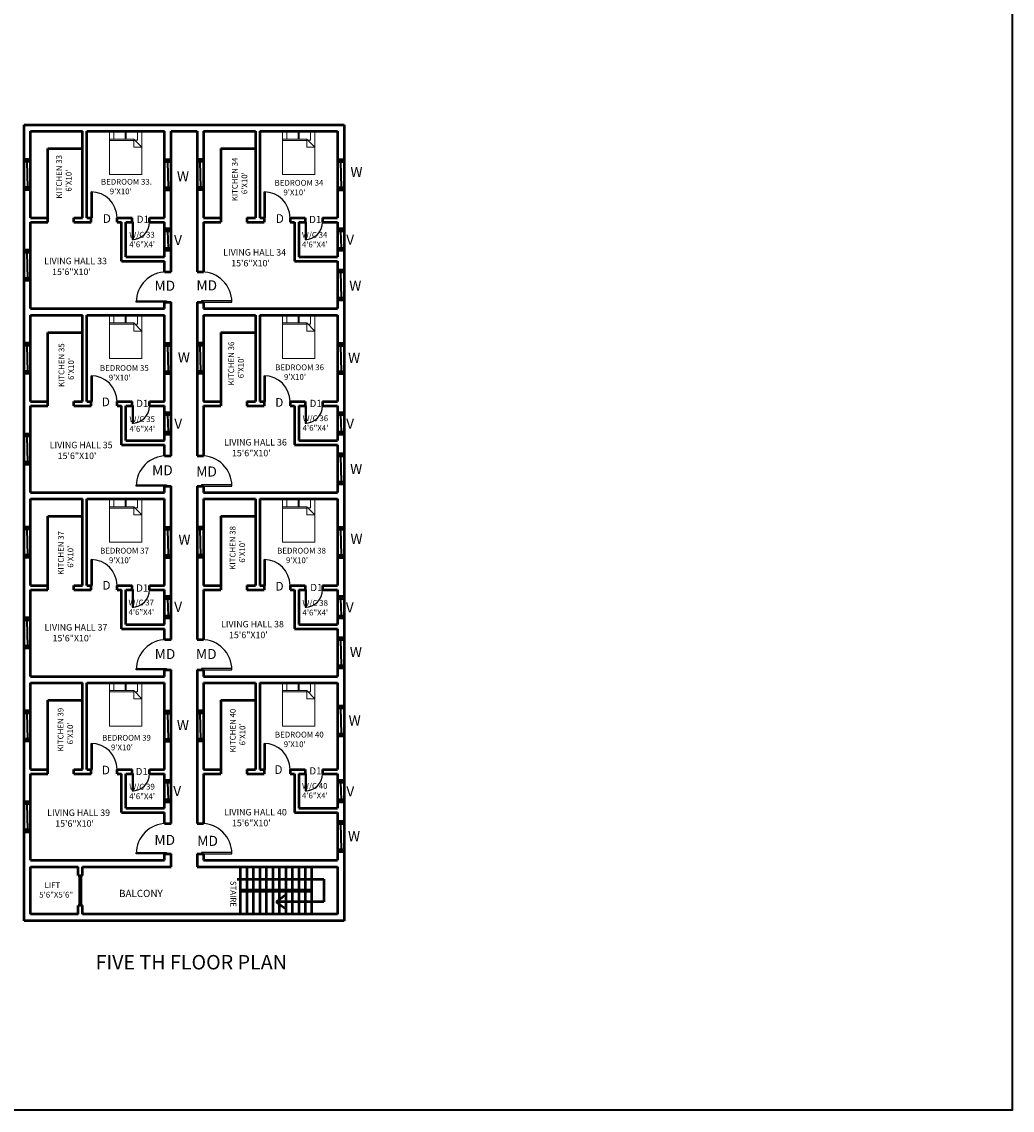
# Model space of a CAD drawing. Units: inches. Extents: x 9239 to 26065, y 6728 to 14611.
# Tile 9 of 12: x 24691 to 26065, y 11592 to 13102. Entities that reach past the tile are written whole.
import ezdxf

# ---------------------------------------------------------------- set-up
doc = ezdxf.new("R2010")
doc.units = ezdxf.units.IN
doc.header["$MEASUREMENT"] = 0
for name, color, linetype, lineweight in [('A-ANNO-TEXT', 7, 'Continuous', 18), ('A-ANNO-TTLB', 7, 'Continuous', 35), ('A-AREA-IDEN', 7, 'Continuous', 18), ('A-DOOR', 4, 'Continuous', 25), ('A-FURN', 8, 'Continuous', 18), ('A-GLAZ', 4, 'Continuous', 25), ('A-WALL', 7, 'Continuous', 50)]:
    doc.layers.add(name, color=color, linetype=linetype, lineweight=lineweight)
doc.styles.get("Standard").update_dxf_attribs({"font": 'arial.ttf'})

# ---------------------------------------------------------------- blocks, each defined once
blk = doc.blocks.new('*U10')
for p, q in [((0, 0), (0, -6)), ((36, 0), (36, -6))]:
    blk.add_line(p, q)
blk.add_lwpolyline([(0, 0), (0, 36), (1.75, 36), (1.75, 0)], close=True)
blk.add_arc((0, 0), 36, 0, 90)
blk = doc.blocks.new('*U34')
for p, q in [((0, 0), (0, 6)), ((24, 0), (24, 6))]:
    blk.add_line(p, q)
blk.add_lwpolyline([(0, 0), (0, -24), (1.75, -24), (1.75, 0)], close=True)
blk.add_arc((0, 0), 24, 270, 0)
blk = doc.blocks.new('*U33')
for p, q in [((-40, 0), (-40, 6)), ((0, 0), (0, 6))]:
    blk.add_line(p, q)
blk.add_lwpolyline([(0, 0), (0, -40), (-1.75, -40), (-1.75, 0)], close=True)
blk.add_arc((0, 0), 40, 180, 270)
blk = doc.blocks.new('*U35')
for p, q in [((0, 0), (0, -6)), ((-40, 0), (-40, -6))]:
    blk.add_line(p, q)
blk.add_lwpolyline([(0, 0), (0, 40), (-1.75, 40), (-1.75, 0)], close=True)
blk.add_arc((0, 0), 40, 90, 180)
blk = doc.blocks.new('Bed - Queen')
for p, q in [((0, -80.00003), (0, 0)), ((0, 0), (59.99999, 0)), ((59.99999, 0), (59.99999, -80.00003)), ((0, -14.4), (44.8, -14.4)), ((44.8, -16.8), (0, -16.8)), ((7.99999, -1.2), (28.79998, -1.2)), ((7.99999, -14.4), (7.99999, -1.2)), ((28.79998, -1.2), (28.79998, -14.4)), ((31.19999, -1.2), (51.99999, -1.2)), ((31.19999, -14.4), (31.19999, -1.2)), ((59.99999, -29.6), (44.8, -14.4)), ((44.8, -14.4), (44.8, -29.6)), ((51.99999, -16.4), (46.79936, -16.4)), ((51.99999, -1.2), (51.99999, -16.4)), ((44.8, -29.6), (59.99999, -29.6)), ((59.99999, -80.00003), (0, -80.00003))]:
    blk.add_line(p, q)
blk = doc.blocks.new('WIN-36')
for p, q in [((0, 1), (36, 1)), ((0, 0.5), (36, 0.5)), ((0, 0), (36, 0))]:
    blk.add_line(p, q)
blk = doc.blocks.new('WIN-24')
for p, q in [((0, 1), (24, 1)), ((0, 0.5), (24, 0.5)), ((0, 0), (24, 0))]:
    blk.add_line(p, q)

msp = doc.modelspace()

# ---------------------------------------------------------------- linework, layer by layer
at = {"layer": 'A-ANNO-TTLB'}
msp.add_lwpolyline([(23324.14, 14611.25), (26064.6, 14611.25), (26064.6, 11591.84), (23324.14, 11591.84)], close=True, dxfattribs=at)
at = {"layer": 'A-WALL'}
for p, q in [((24693.68, 12958.64), (25137.68, 12958.64)), ((24693.68, 11854.64), (24693.68, 12958.64)), ((25137.68, 12958.64), (25137.68, 11854.64)), ((24702.68, 12949.64), (24774.68, 12949.64)), ((24702.68, 12829.64), (24702.68, 12949.64)), ((24774.68, 12829.64), (24774.68, 12949.64)), ((24780.68, 12829.64), (24780.68, 12949.64)), ((24780.68, 12949.64), (24888.68, 12949.64)), ((24888.68, 12829.64), (24888.68, 12949.64)), ((24897.68, 12754.64), (24897.68, 12949.64)), ((24897.68, 12949.64), (24933.68, 12949.64)), ((24933.68, 12949.64), (24933.68, 12754.64)), ((24942.68, 12949.64), (24942.68, 12829.64)), ((24942.68, 12949.64), (25014.68, 12949.64)), ((25014.68, 12949.64), (25014.68, 12829.64)), ((25020.68, 12949.64), (25020.68, 12829.64)), ((25020.68, 12949.64), (25128.68, 12949.64)), ((25128.68, 12949.64), (25128.68, 12829.64)), ((24726.68, 12829.64), (24726.68, 12925.64)), ((24726.68, 12925.64), (24774.68, 12925.64)), ((24966.68, 12925.64), (24966.68, 12829.64)), ((24966.68, 12925.64), (25014.68, 12925.64)), ((24702.68, 12910.64), (24693.68, 12910.64)), ((24888.68, 12910.64), (24897.68, 12910.64)), ((24942.68, 12910.64), (24933.68, 12910.64)), ((25128.68, 12910.64), (25137.68, 12910.64)), ((24702.68, 12907.64), (24693.68, 12907.64)), ((24888.68, 12907.64), (24897.68, 12907.64)), ((24942.68, 12907.64), (24933.68, 12907.64)), ((25128.68, 12907.64), (25137.68, 12907.64)), ((24702.68, 12871.64), (24693.68, 12871.64)), ((24702.68, 12868.64), (24693.68, 12868.64)), ((24888.68, 12871.64), (24897.68, 12871.64)), ((24888.68, 12868.64), (24897.68, 12868.64)), ((24942.68, 12871.64), (24933.68, 12871.64)), ((24942.68, 12868.64), (24933.68, 12868.64)), ((25128.68, 12871.64), (25137.68, 12871.64)), ((25128.68, 12868.64), (25137.68, 12868.64)), ((24702.68, 12829.64), (24726.68, 12829.64)), ((24702.68, 12823.64), (24726.68, 12823.64)), ((24702.68, 12703.64), (24702.68, 12823.64)), ((24726.68, 12823.64), (24726.68, 12829.64)), ((24762.68, 12823.64), (24762.68, 12829.64)), ((24762.68, 12829.64), (24774.68, 12829.64)), ((24762.68, 12823.64), (24786.68, 12823.64)), ((24780.68, 12829.64), (24786.68, 12829.64)), ((24786.68, 12823.64), (24786.68, 12829.64)), ((24822.68, 12823.64), (24822.68, 12829.64)), ((24822.68, 12829.64), (24843.68, 12829.64)), ((24822.68, 12823.64), (24828.68, 12823.64)), ((24828.68, 12769.64), (24828.68, 12823.64)), ((24834.68, 12775.64), (24834.68, 12823.64)), ((24834.68, 12823.64), (24843.68, 12823.64)), ((24843.68, 12823.64), (24843.68, 12829.64)), ((24867.68, 12823.64), (24867.68, 12829.64)), ((24867.68, 12829.64), (24888.68, 12829.64)), ((24867.68, 12823.64), (24888.68, 12823.64)), ((24888.68, 12775.64), (24888.68, 12823.64)), ((24942.68, 12829.64), (24966.68, 12829.64)), ((24942.68, 12823.64), (24966.68, 12823.64)), ((24942.68, 12823.64), (24942.68, 12754.64)), ((24966.68, 12829.64), (24966.68, 12823.64)), ((25002.68, 12829.64), (25002.68, 12823.64)), ((25002.68, 12829.64), (25014.68, 12829.64)), ((25002.68, 12823.64), (25026.68, 12823.64)), ((25020.68, 12829.64), (25026.68, 12829.64)), ((25026.68, 12829.64), (25026.68, 12823.64)), ((25062.68, 12829.64), (25062.68, 12823.64)), ((25062.68, 12829.64), (25083.68, 12829.64)), ((25062.68, 12823.64), (25068.68, 12823.64)), ((25068.68, 12823.64), (25068.68, 12769.64)), ((25074.68, 12823.64), (25074.68, 12775.64)), ((25074.68, 12823.64), (25083.68, 12823.64)), ((25083.68, 12829.64), (25083.68, 12823.64)), ((25107.68, 12829.64), (25107.68, 12823.64)), ((25107.68, 12829.64), (25128.68, 12829.64)), ((25107.68, 12823.64), (25128.68, 12823.64)), ((25128.68, 12823.64), (25128.68, 12775.64)), ((24888.68, 12814.64), (24897.68, 12814.64)), ((24888.68, 12811.64), (24897.68, 12811.64)), ((25128.68, 12814.64), (25137.68, 12814.64)), ((25128.68, 12811.64), (25137.68, 12811.64)), ((24888.68, 12787.64), (24897.68, 12787.64)), ((25128.68, 12787.64), (25137.68, 12787.64)), ((24702.68, 12784.64), (24693.68, 12784.64)), ((24702.68, 12781.64), (24693.68, 12781.64)), ((24834.68, 12775.64), (24888.68, 12775.64)), ((24888.68, 12784.64), (24897.68, 12784.64)), ((25074.68, 12775.64), (25128.68, 12775.64)), ((25128.68, 12784.64), (25137.68, 12784.64)), ((24828.68, 12769.64), (24888.68, 12769.64)), ((24888.68, 12754.64), (24888.68, 12769.64)), ((25068.68, 12769.64), (25128.68, 12769.64)), ((25128.68, 12769.64), (25128.68, 12703.64)), ((25128.68, 12757.64), (25137.68, 12757.64)), ((24702.68, 12745.64), (24693.68, 12745.64)), ((24702.68, 12742.64), (24693.68, 12742.64)), ((24888.68, 12754.64), (24897.68, 12754.64)), ((24933.68, 12754.64), (24942.68, 12754.64)), ((25128.68, 12754.64), (25137.68, 12754.64)), ((24888.68, 12712.64), (24897.68, 12712.64)), ((24888.68, 12703.64), (24888.68, 12712.64)), ((24897.68, 12499.64), (24897.68, 12712.64)), ((24933.68, 12712.64), (24942.68, 12712.64)), ((24933.68, 12712.64), (24933.68, 12499.64)), ((24942.68, 12712.64), (24942.68, 12703.64)), ((25128.68, 12718.64), (25137.68, 12718.64)), ((25128.68, 12715.64), (25137.68, 12715.64)), ((24702.68, 12703.64), (24888.68, 12703.64)), ((24942.68, 12703.64), (25128.68, 12703.64)), ((24702.68, 12694.64), (24774.68, 12694.64)), ((24702.68, 12574.64), (24702.68, 12694.64)), ((24774.68, 12574.64), (24774.68, 12694.64)), ((24780.68, 12574.64), (24780.68, 12694.64)), ((24780.68, 12694.64), (24888.68, 12694.64)), ((24888.68, 12574.64), (24888.68, 12694.64)), ((24942.68, 12694.64), (25014.68, 12694.64)), ((24942.68, 12694.64), (24942.68, 12574.64)), ((25014.68, 12694.64), (25014.68, 12574.64)), ((25020.68, 12694.64), (25020.68, 12574.64)), ((25020.68, 12694.64), (25128.68, 12694.64)), ((25128.68, 12694.64), (25128.68, 12574.64)), ((24726.68, 12574.64), (24726.68, 12670.64)), ((24726.68, 12670.64), (24774.68, 12670.64)), ((24966.68, 12670.64), (24966.68, 12574.64)), ((24966.68, 12670.64), (25014.68, 12670.64)), ((24702.68, 12655.64), (24693.68, 12655.64)), ((24702.68, 12652.64), (24693.68, 12652.64)), ((24888.68, 12655.64), (24897.68, 12655.64)), ((24888.68, 12652.64), (24897.68, 12652.64)), ((24942.68, 12655.64), (24933.68, 12655.64)), ((24942.68, 12652.64), (24933.68, 12652.64)), ((25128.68, 12655.64), (25137.68, 12655.64)), ((25128.68, 12652.64), (25137.68, 12652.64)), ((24702.68, 12616.64), (24693.68, 12616.64)), ((24702.68, 12613.64), (24693.68, 12613.64)), ((24888.68, 12616.64), (24897.68, 12616.64)), ((24888.68, 12613.64), (24897.68, 12613.64)), ((24942.68, 12616.64), (24933.68, 12616.64)), ((24942.68, 12613.64), (24933.68, 12613.64)), ((25128.68, 12616.64), (25137.68, 12616.64)), ((25128.68, 12613.64), (25137.68, 12613.64)), ((24702.68, 12574.64), (24726.68, 12574.64)), ((24702.68, 12568.64), (24726.68, 12568.64)), ((24702.68, 12448.64), (24702.68, 12568.64)), ((24726.68, 12568.64), (24726.68, 12574.64)), ((24762.68, 12568.64), (24762.68, 12574.64)), ((24762.68, 12574.64), (24774.68, 12574.64)), ((24762.68, 12568.64), (24786.68, 12568.64)), ((24780.68, 12574.64), (24786.68, 12574.64)), ((24786.68, 12568.64), (24786.68, 12574.64)), ((24822.68, 12568.64), (24822.68, 12574.64)), ((24822.68, 12574.64), (24843.68, 12574.64)), ((24822.68, 12568.64), (24828.68, 12568.64)), ((24828.68, 12514.64), (24828.68, 12568.64)), ((24834.68, 12520.64), (24834.68, 12568.64)), ((24834.68, 12568.64), (24843.68, 12568.64)), ((24843.68, 12568.64), (24843.68, 12574.64)), ((24867.68, 12568.64), (24867.68, 12574.64)), ((24867.68, 12574.64), (24888.68, 12574.64)), ((24867.68, 12568.64), (24888.68, 12568.64)), ((24888.68, 12520.64), (24888.68, 12568.64)), ((24942.68, 12574.64), (24966.68, 12574.64)), ((24942.68, 12568.64), (24966.68, 12568.64)), ((24942.68, 12568.64), (24942.68, 12499.64)), ((24966.68, 12574.64), (24966.68, 12568.64)), ((25002.68, 12574.64), (25002.68, 12568.64)), ((25002.68, 12574.64), (25014.68, 12574.64)), ((25002.68, 12568.64), (25026.68, 12568.64)), ((25020.68, 12574.64), (25026.68, 12574.64)), ((25026.68, 12574.64), (25026.68, 12568.64)), ((25062.68, 12574.64), (25062.68, 12568.64)), ((25062.68, 12574.64), (25083.68, 12574.64)), ((25062.68, 12568.64), (25068.68, 12568.64)), ((25068.68, 12568.64), (25068.68, 12514.64)), ((25074.68, 12568.64), (25074.68, 12520.64)), ((25074.68, 12568.64), (25083.68, 12568.64)), ((25083.68, 12574.64), (25083.68, 12568.64)), ((25107.68, 12574.64), (25107.68, 12568.64)), ((25107.68, 12574.64), (25128.68, 12574.64)), ((25107.68, 12568.64), (25128.68, 12568.64)), ((25128.68, 12568.64), (25128.68, 12520.64)), ((24888.68, 12559.64), (24897.68, 12559.64)), ((24888.68, 12556.64), (24897.68, 12556.64)), ((25128.68, 12559.64), (25137.68, 12559.64)), ((25128.68, 12556.64), (25137.68, 12556.64)), ((24888.68, 12532.64), (24897.68, 12532.64)), ((25128.68, 12532.64), (25137.68, 12532.64)), ((24702.68, 12529.64), (24693.68, 12529.64)), ((24702.68, 12526.64), (24693.68, 12526.64)), ((24834.68, 12520.64), (24888.68, 12520.64)), ((24888.68, 12529.64), (24897.68, 12529.64)), ((25074.68, 12520.64), (25128.68, 12520.64)), ((25128.68, 12529.64), (25137.68, 12529.64)), ((24828.68, 12514.64), (24888.68, 12514.64)), ((24888.68, 12499.64), (24888.68, 12514.64)), ((25068.68, 12514.64), (25128.68, 12514.64)), ((25128.68, 12514.64), (25128.68, 12448.64)), ((25128.68, 12502.64), (25137.68, 12502.64)), ((24702.68, 12490.64), (24693.68, 12490.64)), ((24702.68, 12487.64), (24693.68, 12487.64)), ((24888.68, 12499.64), (24897.68, 12499.64)), ((24933.68, 12499.64), (24942.68, 12499.64)), ((25128.68, 12499.64), (25137.68, 12499.64)), ((24888.68, 12457.64), (24897.68, 12457.64)), ((24888.68, 12448.64), (24888.68, 12457.64)), ((24897.68, 12244.64), (24897.68, 12457.64)), ((24933.68, 12457.64), (24942.68, 12457.64)), ((24933.68, 12457.64), (24933.68, 12244.64)), ((24942.68, 12457.64), (24942.68, 12448.64)), ((25128.68, 12463.64), (25137.68, 12463.64)), ((25128.68, 12460.64), (25137.68, 12460.64)), ((24702.68, 12448.64), (24888.68, 12448.64)), ((24942.68, 12448.64), (25128.68, 12448.64)), ((24702.68, 12439.64), (24774.68, 12439.64)), ((24702.68, 12319.64), (24702.68, 12439.64)), ((24774.68, 12319.64), (24774.68, 12439.64)), ((24780.68, 12319.64), (24780.68, 12439.64)), ((24780.68, 12439.64), (24888.68, 12439.64)), ((24888.68, 12319.64), (24888.68, 12439.64)), ((24942.68, 12439.64), (25014.68, 12439.64)), ((24942.68, 12439.64), (24942.68, 12319.64)), ((25014.68, 12439.64), (25014.68, 12319.64)), ((25020.68, 12439.64), (25020.68, 12319.64)), ((25020.68, 12439.64), (25128.68, 12439.64)), ((25128.68, 12439.64), (25128.68, 12319.64)), ((24726.68, 12319.64), (24726.68, 12415.64)), ((24726.68, 12415.64), (24774.68, 12415.64)), ((24966.68, 12415.64), (24966.68, 12319.64)), ((24966.68, 12415.64), (25014.68, 12415.64)), ((24702.68, 12400.64), (24693.68, 12400.64)), ((24702.68, 12397.64), (24693.68, 12397.64)), ((24888.68, 12400.64), (24897.68, 12400.64)), ((24888.68, 12397.64), (24897.68, 12397.64)), ((24942.68, 12400.64), (24933.68, 12400.64)), ((24942.68, 12397.64), (24933.68, 12397.64)), ((25128.68, 12400.64), (25137.68, 12400.64)), ((25128.68, 12397.64), (25137.68, 12397.64)), ((24702.68, 12361.64), (24693.68, 12361.64)), ((24702.68, 12358.64), (24693.68, 12358.64)), ((24888.68, 12361.64), (24897.68, 12361.64)), ((24888.68, 12358.64), (24897.68, 12358.64)), ((24942.68, 12361.64), (24933.68, 12361.64)), ((24942.68, 12358.64), (24933.68, 12358.64)), ((25128.68, 12361.64), (25137.68, 12361.64)), ((25128.68, 12358.64), (25137.68, 12358.64)), ((24702.68, 12319.64), (24726.68, 12319.64)), ((24726.68, 12313.64), (24726.68, 12319.64)), ((24762.68, 12313.64), (24762.68, 12319.64)), ((24762.68, 12319.64), (24774.68, 12319.64)), ((24780.68, 12319.64), (24786.68, 12319.64)), ((24786.68, 12313.64), (24786.68, 12319.64)), ((24822.68, 12313.64), (24822.68, 12319.64)), ((24822.68, 12319.64), (24843.68, 12319.64)), ((24843.68, 12313.64), (24843.68, 12319.64)), ((24867.68, 12313.64), (24867.68, 12319.64)), ((24867.68, 12319.64), (24888.68, 12319.64)), ((24942.68, 12319.64), (24966.68, 12319.64)), ((24966.68, 12319.64), (24966.68, 12313.64)), ((25002.68, 12319.64), (25002.68, 12313.64)), ((25002.68, 12319.64), (25014.68, 12319.64)), ((25020.68, 12319.64), (25026.68, 12319.64)), ((25026.68, 12319.64), (25026.68, 12313.64)), ((25062.68, 12319.64), (25062.68, 12313.64)), ((25062.68, 12319.64), (25083.68, 12319.64)), ((25083.68, 12319.64), (25083.68, 12313.64)), ((25107.68, 12319.64), (25107.68, 12313.64)), ((25107.68, 12319.64), (25128.68, 12319.64)), ((24702.68, 12313.64), (24726.68, 12313.64)), ((24702.68, 12193.64), (24702.68, 12313.64)), ((24762.68, 12313.64), (24786.68, 12313.64)), ((24822.68, 12313.64), (24828.68, 12313.64)), ((24828.68, 12259.64), (24828.68, 12313.64)), ((24834.68, 12265.64), (24834.68, 12313.64)), ((24834.68, 12313.64), (24843.68, 12313.64)), ((24867.68, 12313.64), (24888.68, 12313.64)), ((24888.68, 12265.64), (24888.68, 12313.64)), ((24888.68, 12304.64), (24897.68, 12304.64)), ((24942.68, 12313.64), (24966.68, 12313.64)), ((24942.68, 12313.64), (24942.68, 12244.64)), ((25002.68, 12313.64), (25026.68, 12313.64)), ((25062.68, 12313.64), (25068.68, 12313.64)), ((25068.68, 12313.64), (25068.68, 12259.64)), ((25074.68, 12313.64), (25074.68, 12265.64)), ((25074.68, 12313.64), (25083.68, 12313.64)), ((25107.68, 12313.64), (25128.68, 12313.64)), ((25128.68, 12313.64), (25128.68, 12265.64)), ((25128.68, 12304.64), (25137.68, 12304.64)), ((24888.68, 12301.64), (24897.68, 12301.64)), ((25128.68, 12301.64), (25137.68, 12301.64)), ((24702.68, 12274.64), (24693.68, 12274.64)), ((24888.68, 12277.64), (24897.68, 12277.64)), ((24888.68, 12274.64), (24897.68, 12274.64)), ((25128.68, 12277.64), (25137.68, 12277.64)), ((25128.68, 12274.64), (25137.68, 12274.64)), ((24702.68, 12271.64), (24693.68, 12271.64)), ((24828.68, 12259.64), (24888.68, 12259.64)), ((24834.68, 12265.64), (24888.68, 12265.64)), ((24888.68, 12244.64), (24888.68, 12259.64)), ((25068.68, 12259.64), (25128.68, 12259.64)), ((25074.68, 12265.64), (25128.68, 12265.64)), ((25128.68, 12259.64), (25128.68, 12193.64)), ((24888.68, 12244.64), (24897.68, 12244.64)), ((24933.68, 12244.64), (24942.68, 12244.64)), ((25128.68, 12247.64), (25137.68, 12247.64)), ((25128.68, 12244.64), (25137.68, 12244.64)), ((24702.68, 12235.64), (24693.68, 12235.64)), ((24702.68, 12232.64), (24693.68, 12232.64)), ((24888.68, 12202.64), (24897.68, 12202.64)), ((24888.68, 12193.64), (24888.68, 12202.64)), ((24897.68, 11989.64), (24897.68, 12202.64)), ((24933.68, 12202.64), (24942.68, 12202.64)), ((24933.68, 12202.64), (24933.68, 11989.64)), ((24942.68, 12202.64), (24942.68, 12193.64)), ((25128.68, 12208.64), (25137.68, 12208.64)), ((25128.68, 12205.64), (25137.68, 12205.64)), ((24702.68, 12193.64), (24888.68, 12193.64)), ((24702.68, 12184.64), (24774.68, 12184.64)), ((24702.68, 12064.64), (24702.68, 12184.64)), ((24774.68, 12064.64), (24774.68, 12184.64)), ((24780.68, 12064.64), (24780.68, 12184.64)), ((24780.68, 12184.64), (24888.68, 12184.64)), ((24888.68, 12064.64), (24888.68, 12184.64)), ((24942.68, 12193.64), (25128.68, 12193.64)), ((24942.68, 12184.64), (25014.68, 12184.64)), ((24942.68, 12184.64), (24942.68, 12064.64)), ((25014.68, 12184.64), (25014.68, 12064.64)), ((25020.68, 12184.64), (25020.68, 12064.64)), ((25020.68, 12184.64), (25128.68, 12184.64)), ((25128.68, 12184.64), (25128.68, 12064.64)), ((24726.68, 12064.64), (24726.68, 12160.64)), ((24726.68, 12160.64), (24774.68, 12160.64)), ((24966.68, 12160.64), (24966.68, 12064.64)), ((24966.68, 12160.64), (25014.68, 12160.64)), ((24702.68, 12145.64), (24693.68, 12145.64)), ((24702.68, 12142.64), (24693.68, 12142.64)), ((24888.68, 12145.64), (24897.68, 12145.64)), ((24888.68, 12142.64), (24897.68, 12142.64)), ((24942.68, 12145.64), (24933.68, 12145.64)), ((24942.68, 12142.64), (24933.68, 12142.64)), ((25128.68, 12152.9), (25137.68, 12152.9)), ((25128.68, 12149.9), (25137.68, 12149.9)), ((25128.68, 12113.9), (25137.68, 12113.9)), ((25128.68, 12110.9), (25137.68, 12110.9)), ((24702.68, 12106.64), (24693.68, 12106.64)), ((24702.68, 12103.64), (24693.68, 12103.64)), ((24888.68, 12106.64), (24897.68, 12106.64)), ((24888.68, 12103.64), (24897.68, 12103.64)), ((24942.68, 12106.64), (24933.68, 12106.64)), ((24942.68, 12103.64), (24933.68, 12103.64)), ((24702.68, 12064.64), (24726.68, 12064.64)), ((24726.68, 12058.64), (24726.68, 12064.64)), ((24762.68, 12058.64), (24762.68, 12064.64)), ((24762.68, 12064.64), (24774.68, 12064.64)), ((24780.68, 12064.64), (24786.68, 12064.64)), ((24786.68, 12058.64), (24786.68, 12064.64)), ((24822.68, 12058.64), (24822.68, 12064.64)), ((24822.68, 12064.64), (24843.68, 12064.64)), ((24843.68, 12058.64), (24843.68, 12064.64)), ((24867.68, 12058.64), (24867.68, 12064.64)), ((24867.68, 12064.64), (24888.68, 12064.64)), ((24942.68, 12064.64), (24966.68, 12064.64)), ((24966.68, 12064.64), (24966.68, 12058.64)), ((25002.68, 12064.64), (25002.68, 12058.64)), ((25002.68, 12064.64), (25014.68, 12064.64)), ((25020.68, 12064.64), (25026.68, 12064.64)), ((25026.68, 12064.64), (25026.68, 12058.64)), ((25062.68, 12064.64), (25062.68, 12058.64)), ((25062.68, 12064.64), (25083.68, 12064.64)), ((25083.68, 12064.64), (25083.68, 12058.64)), ((25107.68, 12064.64), (25107.68, 12058.64)), ((25107.68, 12064.64), (25128.68, 12064.64)), ((24702.68, 12058.64), (24726.68, 12058.64)), ((24702.68, 11938.64), (24702.68, 12058.64)), ((24762.68, 12058.64), (24786.68, 12058.64)), ((24822.68, 12058.64), (24828.68, 12058.64)), ((24828.68, 12004.64), (24828.68, 12058.64)), ((24834.68, 12010.64), (24834.68, 12058.64)), ((24834.68, 12058.64), (24843.68, 12058.64)), ((24867.68, 12058.64), (24888.68, 12058.64)), ((24888.68, 12010.64), (24888.68, 12058.64)), ((24888.68, 12049.64), (24897.68, 12049.64)), ((24942.68, 12058.64), (24966.68, 12058.64)), ((24942.68, 12058.64), (24942.68, 11989.64)), ((25002.68, 12058.64), (25026.68, 12058.64)), ((25062.68, 12058.64), (25068.68, 12058.64)), ((25068.68, 12058.64), (25068.68, 12004.64)), ((25074.68, 12058.64), (25074.68, 12010.64)), ((25074.68, 12058.64), (25083.68, 12058.64)), ((25107.68, 12058.64), (25128.68, 12058.64)), ((25128.68, 12058.64), (25128.68, 12010.64)), ((25128.68, 12049.64), (25137.68, 12049.64)), ((24888.68, 12046.64), (24897.68, 12046.64)), ((25128.68, 12046.64), (25137.68, 12046.64)), ((24702.68, 12019.64), (24693.68, 12019.64)), ((24888.68, 12022.64), (24897.68, 12022.64)), ((24888.68, 12019.64), (24897.68, 12019.64)), ((25128.68, 12022.64), (25137.68, 12022.64)), ((25128.68, 12019.64), (25137.68, 12019.64)), ((24702.68, 12016.64), (24693.68, 12016.64)), ((24828.68, 12004.64), (24888.68, 12004.64)), ((24834.68, 12010.64), (24888.68, 12010.64)), ((24888.68, 11989.64), (24888.68, 12004.64)), ((25068.68, 12004.64), (25128.68, 12004.64)), ((25074.68, 12010.64), (25128.68, 12010.64)), ((25128.68, 12004.64), (25128.68, 11938.64)), ((24888.68, 11989.64), (24897.68, 11989.64)), ((24933.68, 11989.64), (24942.68, 11989.64)), ((25128.68, 11992.64), (25137.68, 11992.64)), ((25128.68, 11989.64), (25137.68, 11989.64)), ((24702.68, 11980.64), (24693.68, 11980.64)), ((24702.68, 11977.64), (24693.68, 11977.64)), ((24888.68, 11938.64), (24888.68, 11947.64)), ((24888.68, 11947.64), (24897.68, 11947.64)), ((24897.68, 11929.64), (24897.68, 11947.64)), ((24933.68, 11947.64), (24942.68, 11947.64)), ((24933.68, 11947.64), (24933.68, 11929.64)), ((24942.68, 11947.64), (24942.68, 11938.64)), ((25128.68, 11953.64), (25137.68, 11953.64)), ((25128.68, 11950.64), (25137.68, 11950.64)), ((24702.68, 11938.64), (24888.68, 11938.64)), ((24702.68, 11863.64), (24702.68, 11929.64)), ((24702.68, 11929.64), (24768.68, 11929.64)), ((24768.68, 11917.64), (24768.68, 11929.64)), ((24774.68, 11929.64), (24897.68, 11929.64)), ((24774.68, 11917.64), (24774.68, 11929.64)), ((24933.68, 11929.64), (25128.68, 11929.64)), ((24942.68, 11938.64), (25128.68, 11938.64)), ((24993.68, 11929.64), (24993.68, 11863.64)), ((25002.68, 11929.64), (25002.68, 11897.64)), ((25011.68, 11929.64), (25011.68, 11897.64)), ((25020.68, 11929.64), (25020.68, 11897.64)), ((25029.68, 11929.64), (25029.68, 11897.64)), ((25038.68, 11929.64), (25038.68, 11897.64)), ((25047.68, 11929.64), (25047.68, 11897.64)), ((25056.68, 11929.64), (25056.68, 11897.64)), ((25065.68, 11929.64), (25065.68, 11897.64)), ((25074.68, 11929.64), (25074.68, 11897.64)), ((25083.68, 11929.64), (25083.68, 11897.64)), ((25092.68, 11929.64), (25092.68, 11863.64)), ((25128.68, 11929.64), (25128.68, 11863.64)), ((24768.68, 11917.64), (24774.68, 11917.64)), ((24770.68, 11917.64), (24770.68, 11875.64)), ((24772.68, 11917.64), (24772.68, 11875.64)), ((24989.33, 11912.46), (25109.77, 11912.46)), ((25109.77, 11912.46), (25109.77, 11880.96)), ((24993.68, 11897.64), (25092.68, 11897.64)), ((24993.68, 11895.64), (25092.68, 11895.64)), ((25002.68, 11895.64), (25002.68, 11863.64)), ((25011.68, 11895.64), (25011.68, 11863.64)), ((25020.68, 11895.64), (25020.68, 11863.64)), ((25029.68, 11895.64), (25029.68, 11863.64)), ((25038.68, 11895.64), (25038.68, 11863.64)), ((25043.56, 11880.96), (25055.62, 11890.22)), ((25047.68, 11895.64), (25047.68, 11863.64)), ((25056.68, 11895.64), (25056.68, 11863.64)), ((25065.68, 11895.64), (25065.68, 11863.64)), ((25074.68, 11895.64), (25074.68, 11863.64)), ((25083.68, 11895.64), (25083.68, 11863.64)), ((24768.68, 11863.64), (24768.68, 11875.64)), ((24774.68, 11875.64), (24768.68, 11875.64)), ((24774.68, 11863.64), (24774.68, 11875.64)), ((25109.77, 11880.96), (25043.56, 11880.96)), ((25043.56, 11880.96), (25055.34, 11872.2)), ((25137.68, 11854.64), (24693.68, 11854.64)), ((24768.68, 11863.64), (24702.68, 11863.64)), ((25128.68, 11863.64), (24774.68, 11863.64))]:
    msp.add_line(p, q, dxfattribs=at)

# ---------------------------------------------------------------- block references
at = {"layer": 'A-DOOR'}
for name, p in [('*U10', (24786.68, 12829.64)), ('*U10', (25026.68, 12829.64)), ('*U34', (24843.68, 12823.64)), ('*U34', (25083.68, 12823.64)), ('*U10', (24786.68, 12574.64)), ('*U10', (25026.68, 12574.64)), ('*U34', (24843.68, 12568.64)), ('*U34', (25083.68, 12568.64)), ('*U10', (24786.68, 12319.64)), ('*U10', (25026.68, 12319.64)), ('*U34', (24843.68, 12313.64)), ('*U34', (25083.68, 12313.64)), ('*U10', (24786.68, 12064.64)), ('*U10', (25026.68, 12064.64)), ('*U34', (24843.68, 12058.64)), ('*U34', (25083.68, 12058.64))]:
    msp.add_blockref(name, p, dxfattribs=at)
at = {"layer": 'A-DOOR', "xscale": 1.05, "yscale": 1.05, "zscale": 1.05, "rotation": 270}
for name, p in [('*U33', (24891.38, 12712.64)), ('*U35', (24939.98, 12712.64)), ('*U33', (24891.38, 12457.64)), ('*U35', (24939.98, 12457.64)), ('*U33', (24891.38, 12202.64)), ('*U35', (24939.98, 12202.64)), ('*U33', (24891.38, 11947.64)), ('*U35', (24939.98, 11947.64))]:
    msp.add_blockref(name, p, dxfattribs=at)
at = {"layer": 'A-FURN', "xscale": 0.75, "yscale": 0.75, "zscale": 0.75}
for p in [(24812.18, 12949.64), (25052.18, 12949.64), (24812.18, 12694.64), (25052.18, 12694.64), (24812.18, 12439.64), (25052.18, 12439.64), (24812.18, 12184.64), (25052.18, 12184.64)]:
    msp.add_blockref('Bed - Queen', p, dxfattribs=at)
at = {"layer": 'A-GLAZ'}
for name, p, rotation in [('WIN-36', (24697.18, 12907.62), 271.5911402711656), ('WIN-36', (24892.18, 12907.62), 271.5911402712003), ('WIN-36', (24937.18, 12907.62), 271.5911402712003), ('WIN-36', (25132.18, 12907.62), 271.5911402712003), ('WIN-24', (24892.18, 12811.61), 272.3859440303975), ('WIN-24', (25132.18, 12811.61), 272.3859440303975), ('WIN-36', (24697.18, 12781.62), 271.5911402711772), ('WIN-36', (25132.18, 12754.62), 271.5911402712003), ('WIN-36', (24697.18, 12652.62), 271.5911402711772), ('WIN-36', (24892.18, 12652.62), 271.5911402712003), ('WIN-36', (24937.18, 12652.62), 271.5911402711888), ('WIN-36', (25132.18, 12652.62), 271.5911402712003), ('WIN-24', (24892.18, 12556.61), 272.3859440303975), ('WIN-24', (25132.18, 12556.61), 272.3859440303975), ('WIN-36', (24697.18, 12526.62), 271.5911402712003), ('WIN-36', (25132.18, 12499.62), 271.5911402712003), ('WIN-36', (24697.18, 12397.62), 271.5911402712003), ('WIN-36', (24892.18, 12397.62), 271.5911402712003), ('WIN-36', (24937.18, 12397.62), 271.5911402711888), ('WIN-36', (25132.18, 12397.62), 271.5911402712003), ('WIN-24', (24892.18, 12301.61), 272.3859440303975), ('WIN-24', (25132.18, 12301.61), 272.3859440303975), ('WIN-36', (24697.18, 12271.62), 271.5911402712003), ('WIN-36', (25132.18, 12244.62), 271.5911402712003), ('WIN-36', (24697.18, 12142.62), 271.5911402712003), ('WIN-36', (24892.18, 12142.62), 271.5911402712003), ('WIN-36', (24937.18, 12142.62), 271.5911402712003), ('WIN-36', (25132.18, 12149.88), 271.5911402712003), ('WIN-24', (24892.18, 12046.61), 272.3859440303975), ('WIN-24', (25132.18, 12046.61), 272.3859440303975), ('WIN-36', (24697.18, 12016.62), 271.5911402712003), ('WIN-36', (25132.18, 11989.62), 271.5911402712003)]:
    msp.add_blockref(name, p, dxfattribs=dict(at, rotation=rotation))

# ---------------------------------------------------------------- texts
at = {"layer": 'A-ANNO-TEXT', "attachment_point": 1}
for s, width, insert, char_height in [('W', 545.3335, (24905.8, 12894.23), 14), ('W', 545.3335, (25146.48, 12900.21), 14), ('D', 545.3335, (24802.98, 12834.66), 12), ('D1', 545.3335, (24850.01, 12832.53), 10), ('D', 545.3335, (25042.86, 12834.65), 12), ('D1', 545.3335, (25089.23, 12832.36), 10), ('W/C 33\\P4\'6"X4\'', 1026.6179, (24839.65, 12810.14), 8), ('V', 545.3335, (24901.79, 12805.72), 14), ('W/C 34\\P4\'6"X4\'', 1026.6179, (25079.16, 12809.97), 8), ('V', 545.3335, (25140.6, 12806.47), 14), ('MD', 545.3335, (24874.62, 12742.44), 14), ('MD', 545.3335, (24932.83, 12742.94), 14), ('W', 545.3335, (25144.87, 12742.55), 14), ('W', 545.3335, (24907.08, 12643.04), 14), ('W', 545.3335, (25143.24, 12642.48), 14), ('D', 545.3335, (24801.5, 12580.35), 12), ('D1', 545.3335, (24849.27, 12577.19), 10), ('D', 545.3335, (25042.16, 12579.56), 12), ('D1', 545.3335, (25089.9, 12577.22), 10), ('W/C 35\\P4\'6"X4\'', 1026.6179, (24839.88, 12554.34), 8), ('V', 545.3335, (24902.08, 12551.1), 14), ('W/C 36\\P4\'6"X4\'', 1026.6179, (25080.2, 12555.58), 8), ('V', 545.3335, (25140.56, 12551.25), 14), ('MD', 545.3335, (24871.29, 12486.45), 14), ('W', 545.3335, (25146.1, 12488.39), 14), ('MD', 545.3335, (24932.58, 12484.73), 14), ('W', 545.3335, (24907.88, 12390.31), 14), ('W', 545.3335, (25146.51, 12391.4), 14), ('D', 545.3335, (24802.42, 12325.9), 12), ('D1', 545.3335, (24849.23, 12321.19), 10), ('D', 545.3335, (25042.5, 12324.59), 12), ('D1', 545.3335, (25090.76, 12321.85), 10), ('W/C 37\\P4\'6"X4\'', 1026.6179, (24838.6, 12300), 8), ('V', 545.3335, (24901.96, 12296.99), 14), ('W/C 38\\P4\'6"X4\'', 1026.6179, (25079.92, 12299.46), 8), ('V', 545.3335, (25140.06, 12296.32), 14), ('MD', 545.3335, (24874.92, 12231.62), 14), ('MD', 545.3335, (24932.18, 12231.62), 14), ('W', 545.3335, (25145.64, 12234.27), 14), ('W', 545.3335, (25144.01, 12139.4), 14), ('W', 545.3335, (24905.7, 12133.02), 14), ('D', 545.3335, (24801.54, 12069.67), 12), ('D1', 545.3335, (24848.53, 12066.65), 10), ('D', 545.3335, (25040.98, 12070.3), 12), ('D1', 545.3335, (25089.5, 12067.51), 10), ('W/C 39\\P4\'6"X4\'', 1026.6179, (24839.66, 12044.6), 8), ('V', 545.3335, (24900.71, 12041.68), 14), ('W/C 40\\P4\'6"X4\'', 1026.6179, (25079.28, 12045.69), 8), ('V', 545.3335, (25140.8, 12041.24), 14), ('MD', 545.3335, (24874.56, 11973.73), 14), ('MD', 545.3335, (24934.04, 11972.45), 14), ('W', 545.3335, (25143.1, 11978.91), 14), ('   LIFT\\P5\'6"X5\'6"', 441.5638, (24714.82, 11908.07), 8), ('FIVE TH FLOOR PLAN', 1203.1671, (24792.9, 11807.15), 20)]:
    msp.add_mtext_dynamic_manual_height_columns(s, width=width, gutter_width=1, heights=[0], dxfattribs=dict(at, insert=insert, char_height=char_height))
at = {"layer": 'A-AREA-IDEN', "char_height": 8, "attachment_point": 1}
for s, width, insert, rotation in [("KITCHEN 33\\P    6'X10'", 757.9977, (24738.3, 12856.17), 90), ("KITCHEN 34\\P    6'X10'", 757.9977, (24982.09, 12852.62), 90), ("KITCHEN 35\\P    6'X10'", 757.9977, (24741.61, 12594.98), 90), ("KITCHEN 36\\P    6'X10'", 757.9977, (24977.17, 12597.25), 90), ("KITCHEN 38\\P    6'X10'", 757.9977, (24979.03, 12341.52), 90), ("KITCHEN 37\\P    6'X10'", 757.9977, (24740.79, 12334.55), 90), ("KITCHEN 39\\P    6'X10'", 757.9977, (24740.39, 12089.43), 90), ("KITCHEN 40\\P    6'X10'", 757.9977, (24979.27, 12088.09), 90), ('STAIRE', 294.5156, (24987.98, 11909.97), 270)]:
    msp.add_mtext_dynamic_manual_height_columns(s, width=width, gutter_width=1, heights=[0], dxfattribs=dict(at, insert=insert, rotation=rotation))
at = {"layer": 'A-AREA-IDEN', "attachment_point": 1}
for s, width, insert, char_height in [("BEDROOM 33.\\P     9'X10'", 562.7126, (24800.39, 12883.59), 8), ("BEDROOM 34\\P     9'X10'", 562.7126, (25041.26, 12882.22), 8), ('LIVING HALL 33\\P    15\'6"X10\'', 436.6568, (24721.64, 12774.23), 9), ('LIVING HALL 34\\P    15\'6"X10\'', 436.6568, (24970.07, 12786.22), 9), ("BEDROOM 35\\P     9'X10'", 562.7126, (24798.98, 12625.37), 8), ("BEDROOM 36\\P     9'X10'", 562.7126, (25042.14, 12626.22), 8), ('LIVING HALL 35\\P    15\'6"X10\'', 436.6568, (24729.38, 12519.01), 9), ('LIVING HALL 36\\P    15\'6"X10\'', 436.6568, (24971.12, 12522.78), 9), ("BEDROOM 37\\P     9'X10'", 562.7126, (24799.26, 12371.95), 8), ("BEDROOM 38\\P     9'X10'", 562.7126, (25044.87, 12371.95), 8), ('LIVING HALL 37\\P    15\'6"X10\'', 436.6568, (24722.19, 12266.11), 9), ('LIVING HALL 38\\P    15\'6"X10\'', 436.6568, (24967.06, 12270.55), 9), ("BEDROOM 39\\P     9'X10'", 562.7126, (24802, 12112.42), 8), ("BEDROOM 40\\P     9'X10'", 562.7126, (25041.74, 12116.81), 8), ('LIVING HALL 39\\P    15\'6"X10\'', 436.6568, (24725.9, 12008.97), 9), ('LIVING HALL 40\\P    15\'6"X10\'', 436.6568, (24971.11, 12009.73), 9), ('BALCONY', 294.5156, (24825.48, 11897.55), 10)]:
    msp.add_mtext_dynamic_manual_height_columns(s, width=width, gutter_width=1, heights=[0], dxfattribs=dict(at, insert=insert, char_height=char_height))

doc.saveas('drawing.dxf')
